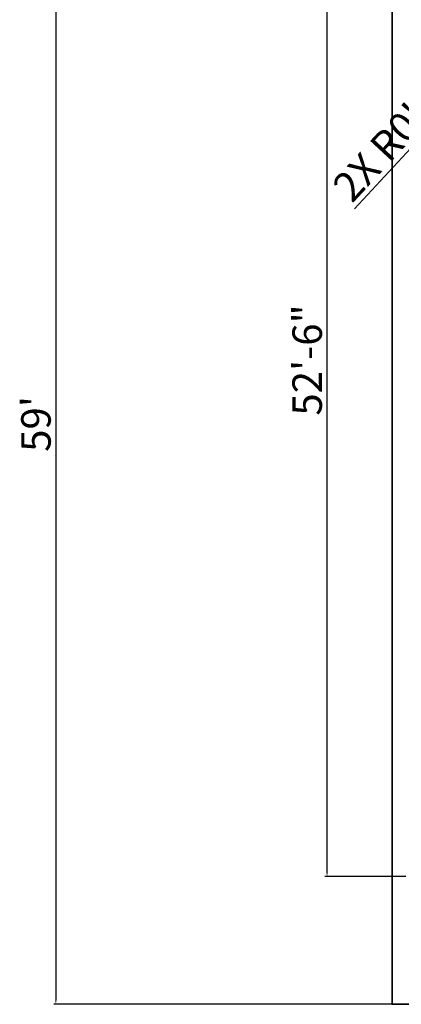
# Model space of a CAD drawing. Units: inches. Extents: x 2040 to 2729, y 1653 to 2621.
# Tile 1 of 4: x 2040 to 2273, y 1695 to 2295. Entities that reach past the tile are written whole.
import ezdxf

# ---------------------------------------------------------------- set-up
doc = ezdxf.new("R2010")
doc.units = ezdxf.units.IN
doc.layers.add('A-ANNO-DIMS', color=10, linetype='Continuous', lineweight=18)
doc.layers.add('C-PROP', color=111, linetype='Continuous', lineweight=35)
doc.styles.get("Standard").update_dxf_attribs({"font": 'arial.ttf'})
doc.dimstyles.new('ISO-25', dxfattribs={"dimtxt": 18, "dimasz": 2.5, "dimexe": 1.25, "dimexo": 0.625, "dimtad": 1, "dimdec": 0, "dimlunit": 3, "dimtxsty": 'Standard', "dimcen": 2.5, "dimadec": 0, "dimazin": 0, "dimtfac": 1, "dimtdec": 0, "dimtmove": 0, "dimatfit": 3, "dimfxl": 1, "dimarcsym": 0})

# ---------------------------------------------------------------- blocks, each defined once
blk = doc.blocks.new('*D5')
at = {"layer": 'A-ANNO-DIMS', "color": 0, "lineweight": -2, "transparency": 16777216}
for p, q in [((2266.85, 2402.66), (2060.98, 2402.66)), ((2062.23, 2400.16), (2062.23, 1697.16)), ((2266.85, 1694.66), (2060.98, 1694.66))]:
    blk.add_line(p, q, dxfattribs=at)
at = {"layer": 'A-ANNO-DIMS', "color": 0, "transparency": 16777216}
for points in [[(2061.81, 2400.16), (2062.64, 2400.16), (2062.23, 2402.66)], [(2061.81, 1697.16), (2062.64, 1697.16), (2062.23, 1694.66)]]:
    blk.add_solid(points, dxfattribs=at)
at = {"layer": 'Defpoints', "color": 0, "transparency": 16777216}
for p in [(2267.47, 2402.66), (2062.23, 1694.66), (2267.47, 1694.66)]:
    blk.add_point(p, dxfattribs=at)
at = {"layer": 'A-ANNO-DIMS', "color": 0, "transparency": 16777216, "insert": (2052.41, 2048.66), "char_height": 18, "attachment_point": 5, "rotation": 90}
blk.add_mtext("59'", dxfattribs=at)
blk = doc.blocks.new('*D41')
at = {"layer": 'A-ANNO-DIMS', "color": 0, "lineweight": -2, "transparency": 16777216}
for p, q in [((2266.85, 2402.66), (2226.49, 2402.66)), ((2227.74, 1775.16), (2227.74, 2400.16)), ((2275.85, 1772.66), (2226.49, 1772.66))]:
    blk.add_line(p, q, dxfattribs=at)
at = {"layer": 'A-ANNO-DIMS', "color": 0, "transparency": 16777216}
for points in [[(2227.33, 2400.16), (2228.16, 2400.16), (2227.74, 2402.66)], [(2227.33, 1775.16), (2228.16, 1775.16), (2227.74, 1772.66)]]:
    blk.add_solid(points, dxfattribs=at)
at = {"layer": 'Defpoints', "color": 0, "transparency": 16777216}
for p in [(2227.74, 2402.66), (2267.47, 2402.66), (2276.47, 1772.66)]:
    blk.add_point(p, dxfattribs=at)
at = {"layer": 'A-ANNO-DIMS', "color": 0, "transparency": 16777216, "insert": (2217.93, 2087.66), "char_height": 18, "attachment_point": 5, "rotation": 90}
blk.add_mtext('52\'-6"', dxfattribs=at)
blk = doc.blocks.new('*D50')
at = {"layer": 'A-ANNO-DIMS', "color": 0, "lineweight": -2, "transparency": 16777216}
for p, q in [((2335.72, 2278.24), (2328.94, 2270.92)), ((2244.45, 2179.76), (2327.24, 2269.09))]:
    blk.add_line(p, q, dxfattribs=at)
at = {"layer": 'A-ANNO-DIMS', "color": 0, "transparency": 16777216}
blk.add_solid([(2326.93, 2269.37), (2327.54, 2268.81), (2328.94, 2270.92)], dxfattribs=at)
at = {"layer": 'Defpoints', "color": 0, "transparency": 16777216}
for p in [(2335.72, 2278.24), (2328.94, 2270.92)]:
    blk.add_point(p, dxfattribs=at)
at = {"layer": 'A-ANNO-DIMS', "color": 0, "transparency": 16777216, "insert": (2277.8, 2230.18), "char_height": 18, "attachment_point": 5, "rotation": 47.17513}
blk.add_mtext('2X R0\'-10"', dxfattribs=at)

msp = doc.modelspace()

# ---------------------------------------------------------------- linework, layer by layer
at = {"layer": 'C-PROP'}
msp.add_lwpolyline([(2267.47, 2402.66), (2621.47, 2402.66), (2621.47, 1694.66), (2267.47, 1694.66)], close=True, dxfattribs=at)

# ---------------------------------------------------------------- dimensions: what is measured, and where the dimension line sits
at = {"layer": 'A-ANNO-DIMS'}
for base, p1, p2, override, picture, middle in [((2062.23, 1694.66), (2267.47, 2402.66), (2267.47, 1694.66), {"dimclrd": 0, "dimclre": 0, "dimclrt": 0}, '*D5', (2052.41, 2048.66)), ((2227.74, 2402.66), (2276.47, 1772.66), (2267.47, 2402.66), {"dimdec": 1, "dimlfac": 1, "dimrnd": 0, "dimzin": 1, "dimdsep": 46, "dimlunit": 4, "dimfrac": 2}, '*D41', (2217.93, 2087.66))]:
    dim = msp.add_linear_dim(base=base, p1=p1, p2=p2, angle=90, dimstyle='ISO-25', override=override, dxfattribs=at)
    dim.commit()
    dim.dimension.update_dxf_attribs({"geometry": picture, "text_midpoint": middle})
dim = msp.add_radius_dim(center=(2335.72, 2278.24), mpoint=(2328.94, 2270.92), text='2X <>', dimstyle='ISO-25', override={"dimdec": 1, "dimlfac": 1, "dimrnd": 0, "dimzin": 1, "dimdsep": 46, "dimlunit": 4, "dimfrac": 2}, dxfattribs=at)
dim.commit()
dim.dimension.update_dxf_attribs({"geometry": '*D50', "text_midpoint": (2277.8, 2230.18)})

doc.saveas('drawing.dxf')
